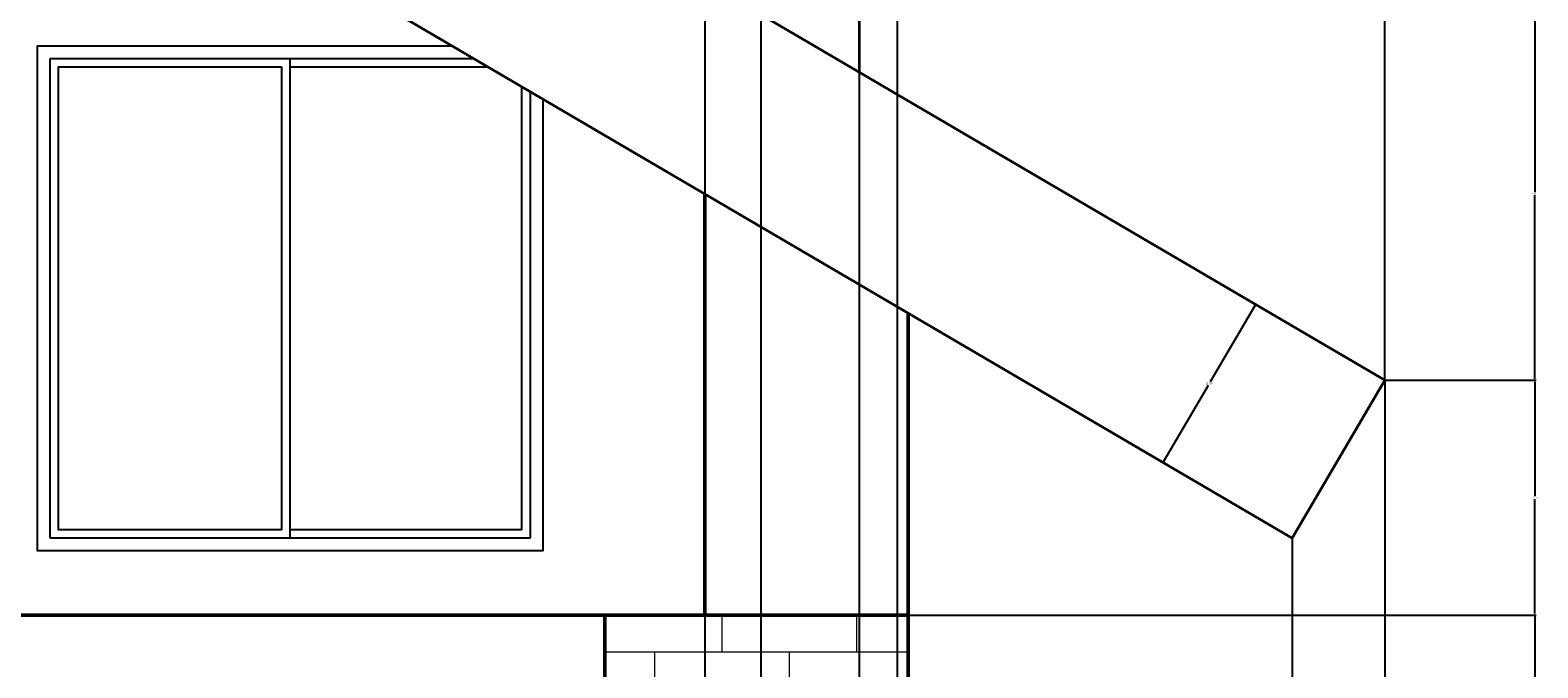
# Model space of a CAD drawing. Units: inches. Extents: x 27 to 409, y -26 to 294.
# Tile 6 of 7: x 230 to 409, y 102 to 178. Entities that reach past the tile are written whole.
import ezdxf

# ---------------------------------------------------------------- set-up
doc = ezdxf.new("R2010")
doc.units = ezdxf.units.IN
doc.header["$MEASUREMENT"] = 0
for name, color, linetype, lineweight in [('A-ANNO-DIMS', 2, 'Continuous', 18), ('A-GLAZ', 4, 'Continuous', 25), ('A-ROOF', 1, 'Continuous', 35), ('A-WALL', 7, 'Continuous', 50), ('A-WALL-PATT', 8, 'Continuous', 13)]:
    doc.layers.add(name, color=color, linetype=linetype, lineweight=lineweight)
doc.styles.get("Standard").update_dxf_attribs({"font": 'arial.ttf'})
doc.dimstyles.get("Standard").update_dxf_attribs({"dimtxt": 0.18, "dimasz": 0.18, "dimexe": 0.18, "dimexo": 0.0625, "dimgap": 0.09, "dimtad": 0, "dimtih": 1, "dimtoh": 1, "dimdec": 4, "dimzin": 0, "dimdsep": 46, "dimtxsty": 'Standard', "dimcen": 0.09, "dimadec": 0, "dimazin": 0, "dimtfac": 1, "dimtdec": 4, "dimtofl": 0, "dimtmove": 0, "dimatfit": 3, "dimfxl": 1, "dimtolj": 1, "dimtzin": 0, "dimarcsym": 0})

# ---------------------------------------------------------------- blocks, each defined once
blk = doc.blocks.new('*D7')
at = {"layer": 'A-ANNO-DIMS', "color": 0, "lineweight": -2, "transparency": 16777216}
for p, q in [((45.58, 108.44), (45.58, 293.63)), ((45.76, 293.45), (217.77, 293.45)), ((390.53, 293.45), (218.52, 293.45)), ((390.71, 136.32), (390.71, 293.63))]:
    blk.add_line(p, q, dxfattribs=at)
at = {"layer": 'A-ANNO-DIMS', "color": 0, "transparency": 16777216}
for points in [[(45.76, 293.48), (45.76, 293.42), (45.58, 293.45)], [(390.53, 293.48), (390.53, 293.42), (390.71, 293.45)]]:
    blk.add_solid(points, dxfattribs=at)
at = {"layer": 'Defpoints', "color": 0, "transparency": 16777216}
for p in [(390.71, 293.45), (390.71, 136.26), (45.58, 108.38)]:
    blk.add_point(p, dxfattribs=at)
at = {"layer": 'A-ANNO-DIMS', "color": 0, "transparency": 16777216, "insert": (218.14, 293.45), "char_height": 0.18, "attachment_point": 5}
blk.add_mtext('\\A1;345.1', dxfattribs=at)
blk = doc.blocks.new('*D20')
at = {"layer": 'A-ANNO-DIMS', "color": 0, "lineweight": -2, "transparency": 16777216}
for p, q in [((210.09, 143.71), (210.09, -26.5)), ((230.52, -8.58), (230.52, -26.5)), ((210.27, -26.32), (219.84, -26.32)), ((230.34, -26.32), (220.77, -26.32))]:
    blk.add_line(p, q, dxfattribs=at)
at = {"layer": 'A-ANNO-DIMS', "color": 0, "transparency": 16777216}
for points in [[(210.27, -26.29), (210.27, -26.35), (210.09, -26.32)], [(230.34, -26.29), (230.34, -26.35), (230.52, -26.32)]]:
    blk.add_solid(points, dxfattribs=at)
at = {"layer": 'Defpoints', "color": 0, "transparency": 16777216}
for p in [(210.09, 143.77), (230.52, -8.52), (230.52, -26.32)]:
    blk.add_point(p, dxfattribs=at)
at = {"layer": 'A-ANNO-DIMS', "color": 0, "transparency": 16777216, "insert": (220.31, -26.32), "char_height": 0.18, "attachment_point": 5}
blk.add_mtext('\\A1;20.435', dxfattribs=at)
blk = doc.blocks.new('*D21')
at = {"layer": 'A-ANNO-DIMS', "color": 0, "lineweight": -2, "transparency": 16777216}
for p, q in [((298.08, 108.32), (298.08, -26.5)), ((230.52, -8.58), (230.52, -26.5)), ((230.7, -26.32), (263.9, -26.32)), ((297.9, -26.32), (264.69, -26.32))]:
    blk.add_line(p, q, dxfattribs=at)
at = {"layer": 'A-ANNO-DIMS', "color": 0, "transparency": 16777216}
for points in [[(230.7, -26.29), (230.7, -26.35), (230.52, -26.32)], [(297.9, -26.29), (297.9, -26.35), (298.08, -26.32)]]:
    blk.add_solid(points, dxfattribs=at)
at = {"layer": 'Defpoints', "color": 0, "transparency": 16777216}
for p in [(298.08, 108.38), (230.52, -8.52), (298.08, -26.32)]:
    blk.add_point(p, dxfattribs=at)
at = {"layer": 'A-ANNO-DIMS', "color": 0, "transparency": 16777216, "insert": (264.3, -26.32), "char_height": 0.18, "attachment_point": 5}
blk.add_mtext('\\A1;67.55', dxfattribs=at)
blk = doc.blocks.new('*D22')
at = {"layer": 'A-ANNO-DIMS', "color": 0, "lineweight": -2, "transparency": 16777216}
for p, q in [((309.93, 158.34), (309.93, -26.5)), ((298.08, 108.32), (298.08, -26.5)), ((298.26, -26.32), (303.61, -26.32)), ((309.75, -26.32), (304.39, -26.32))]:
    blk.add_line(p, q, dxfattribs=at)
at = {"layer": 'A-ANNO-DIMS', "color": 0, "transparency": 16777216}
for points in [[(298.26, -26.29), (298.26, -26.35), (298.08, -26.32)], [(309.75, -26.29), (309.75, -26.35), (309.93, -26.32)]]:
    blk.add_solid(points, dxfattribs=at)
at = {"layer": 'Defpoints', "color": 0, "transparency": 16777216}
for p in [(309.93, 158.4), (298.08, 108.38), (309.93, -26.32)]:
    blk.add_point(p, dxfattribs=at)
at = {"layer": 'A-ANNO-DIMS', "color": 0, "transparency": 16777216, "insert": (304, -26.32), "char_height": 0.18, "attachment_point": 5}
blk.add_mtext('\\A1;11.85', dxfattribs=at)
blk = doc.blocks.new('*D23')
at = {"layer": 'A-ANNO-DIMS', "color": 0, "lineweight": -2, "transparency": 16777216}
for p, q in [((309.93, 158.34), (309.93, -26.5)), ((334.08, 15.42), (334.08, -26.5)), ((310.11, -26.32), (321.6, -26.32)), ((333.9, -26.32), (322.4, -26.32))]:
    blk.add_line(p, q, dxfattribs=at)
at = {"layer": 'A-ANNO-DIMS', "color": 0, "transparency": 16777216}
for points in [[(310.11, -26.29), (310.11, -26.35), (309.93, -26.32)], [(333.9, -26.29), (333.9, -26.35), (334.08, -26.32)]]:
    blk.add_solid(points, dxfattribs=at)
at = {"layer": 'Defpoints', "color": 0, "transparency": 16777216}
for p in [(309.93, 158.4), (334.08, 15.48), (334.08, -26.32)]:
    blk.add_point(p, dxfattribs=at)
at = {"layer": 'A-ANNO-DIMS', "color": 0, "transparency": 16777216, "insert": (322, -26.32), "char_height": 0.18, "attachment_point": 5}
blk.add_mtext('\\A1;24.15', dxfattribs=at)
blk = doc.blocks.new('*D24')
at = {"layer": 'A-ANNO-DIMS', "color": 0, "lineweight": -2, "transparency": 16777216}
for p, q in [((379.72, 117.44), (379.72, -26.5)), ((334.08, 15.42), (334.08, -26.5)), ((334.26, -26.32), (356.5, -26.32)), ((379.54, -26.32), (357.29, -26.32))]:
    blk.add_line(p, q, dxfattribs=at)
at = {"layer": 'A-ANNO-DIMS', "color": 0, "transparency": 16777216}
for points in [[(334.26, -26.29), (334.26, -26.35), (334.08, -26.32)], [(379.54, -26.29), (379.54, -26.35), (379.72, -26.32)]]:
    blk.add_solid(points, dxfattribs=at)
at = {"layer": 'Defpoints', "color": 0, "transparency": 16777216}
for p in [(379.72, 117.5), (334.08, 15.48), (379.72, -26.32)]:
    blk.add_point(p, dxfattribs=at)
at = {"layer": 'A-ANNO-DIMS', "color": 0, "transparency": 16777216, "insert": (356.9, -26.32), "char_height": 0.18, "attachment_point": 5}
blk.add_mtext('\\A1;45.64', dxfattribs=at)
blk = doc.blocks.new('*D25')
at = {"layer": 'A-ANNO-DIMS', "color": 0, "lineweight": -2, "transparency": 16777216}
for p, q in [((390.71, 136.19), (390.71, -26.5)), ((379.72, 117.44), (379.72, -26.5)), ((379.9, -26.32), (384.83, -26.32)), ((390.53, -26.32), (385.6, -26.32))]:
    blk.add_line(p, q, dxfattribs=at)
at = {"layer": 'A-ANNO-DIMS', "color": 0, "transparency": 16777216}
for points in [[(379.9, -26.29), (379.9, -26.35), (379.72, -26.32)], [(390.53, -26.29), (390.53, -26.35), (390.71, -26.32)]]:
    blk.add_solid(points, dxfattribs=at)
at = {"layer": 'Defpoints', "color": 0, "transparency": 16777216}
for p in [(390.71, 136.26), (379.72, 117.5), (390.71, -26.32)]:
    blk.add_point(p, dxfattribs=at)
at = {"layer": 'A-ANNO-DIMS', "color": 0, "transparency": 16777216, "insert": (385.21, -26.32), "char_height": 0.18, "attachment_point": 5}
blk.add_mtext('\\A1;10.99', dxfattribs=at)
blk = doc.blocks.new('*D42')
at = {"layer": 'A-ANNO-DIMS', "color": 0, "lineweight": -2, "transparency": 16777216}
for p, q in [((334.14, 108.38), (408.69, 108.38)), ((408.51, 108.2), (408.51, 62.11)), ((408.51, 15.66), (408.51, 61.75)), ((334.14, 15.48), (408.69, 15.48))]:
    blk.add_line(p, q, dxfattribs=at)
at = {"layer": 'A-ANNO-DIMS', "color": 0, "transparency": 16777216}
for points in [[(408.48, 108.2), (408.54, 108.2), (408.51, 108.38)], [(408.48, 15.66), (408.54, 15.66), (408.51, 15.48)]]:
    blk.add_solid(points, dxfattribs=at)
at = {"layer": 'Defpoints', "color": 0, "transparency": 16777216}
for p in [(334.08, 108.38), (408.51, 108.38), (334.08, 15.48)]:
    blk.add_point(p, dxfattribs=at)
at = {"layer": 'A-ANNO-DIMS', "color": 0, "transparency": 16777216, "insert": (408.51, 61.93), "char_height": 0.18, "attachment_point": 5}
blk.add_mtext('\\A1;92.9', dxfattribs=at)
blk = doc.blocks.new('*D43')
at = {"layer": 'A-ANNO-DIMS', "color": 0, "lineweight": -2, "transparency": 16777216}
for p, q in [((390.77, 136.26), (408.69, 136.26)), ((408.51, 136.08), (408.51, 122.5)), ((408.51, 108.56), (408.51, 122.14)), ((334.14, 108.38), (408.69, 108.38))]:
    blk.add_line(p, q, dxfattribs=at)
at = {"layer": 'A-ANNO-DIMS', "color": 0, "transparency": 16777216}
for points in [[(408.48, 136.08), (408.54, 136.08), (408.51, 136.26)], [(408.48, 108.56), (408.54, 108.56), (408.51, 108.38)]]:
    blk.add_solid(points, dxfattribs=at)
at = {"layer": 'Defpoints', "color": 0, "transparency": 16777216}
for p in [(390.71, 136.26), (408.51, 136.26), (334.08, 108.38)]:
    blk.add_point(p, dxfattribs=at)
at = {"layer": 'A-ANNO-DIMS', "color": 0, "transparency": 16777216, "insert": (408.51, 122.32), "char_height": 0.18, "attachment_point": 5}
blk.add_mtext('\\A1;27.877', dxfattribs=at)
blk = doc.blocks.new('*D44')
at = {"layer": 'A-ANNO-DIMS', "color": 0, "lineweight": -2, "transparency": 16777216}
for p, q in [((166.14, 180.59), (408.69, 180.59)), ((408.51, 180.41), (408.51, 158.6)), ((408.51, 136.44), (408.51, 158.24)), ((390.77, 136.26), (408.69, 136.26))]:
    blk.add_line(p, q, dxfattribs=at)
at = {"layer": 'A-ANNO-DIMS', "color": 0, "transparency": 16777216}
for points in [[(408.48, 180.41), (408.54, 180.41), (408.51, 180.59)], [(408.48, 136.44), (408.54, 136.44), (408.51, 136.26)]]:
    blk.add_solid(points, dxfattribs=at)
at = {"layer": 'Defpoints', "color": 0, "transparency": 16777216}
for p in [(166.08, 180.59), (408.51, 180.59), (390.71, 136.26)]:
    blk.add_point(p, dxfattribs=at)
at = {"layer": 'A-ANNO-DIMS', "color": 0, "transparency": 16777216, "insert": (408.51, 158.42), "char_height": 0.18, "attachment_point": 5}
blk.add_mtext('\\A1;44.33', dxfattribs=at)
blk = doc.blocks.new('*D52')
at = {"layer": 'A-ANNO-DIMS', "color": 0, "lineweight": -2, "transparency": 16777216}
for p, q in [((375.26, 145.1), (369.96, 136.06)), ((390.65, 136.29), (375.19, 145.35)), ((364.45, 126.66), (369.75, 135.7)), ((379.66, 117.54), (364.2, 126.59))]:
    blk.add_line(p, q, dxfattribs=at)
at = {"layer": 'A-ANNO-DIMS', "color": 0, "transparency": 16777216}
for points in [[(375.23, 145.12), (375.28, 145.09), (375.35, 145.26)], [(364.42, 126.67), (364.48, 126.64), (364.36, 126.5)]]:
    blk.add_solid(points, dxfattribs=at)
at = {"layer": 'Defpoints', "color": 0, "transparency": 16777216}
for p in [(375.35, 145.26), (390.71, 136.26), (379.72, 117.5)]:
    blk.add_point(p, dxfattribs=at)
at = {"layer": 'A-ANNO-DIMS', "color": 0, "transparency": 16777216, "insert": (369.85, 135.88), "char_height": 0.18, "attachment_point": 5}
blk.add_mtext('\\A1;21.736', dxfattribs=at)
blk = doc.blocks.new('*D82')
at = {"layer": 'A-ANNO-DIMS', "color": 0, "lineweight": -2, "transparency": 16777216}
for p, q in [((309.93, 228.32), (309.93, -26.5)), ((316.59, 228.32), (316.59, -26.5)), ((310.11, -26.32), (312.86, -26.32)), ((316.41, -26.32), (313.65, -26.32))]:
    blk.add_line(p, q, dxfattribs=at)
at = {"layer": 'A-ANNO-DIMS', "color": 0, "transparency": 16777216}
for points in [[(310.11, -26.29), (310.11, -26.35), (309.93, -26.32)], [(316.41, -26.29), (316.41, -26.35), (316.59, -26.32)]]:
    blk.add_solid(points, dxfattribs=at)
at = {"layer": 'Defpoints', "color": 0, "transparency": 16777216}
for p in [(309.93, 228.38), (316.59, 228.38), (316.59, -26.32)]:
    blk.add_point(p, dxfattribs=at)
at = {"layer": 'A-ANNO-DIMS', "color": 0, "transparency": 16777216, "insert": (313.26, -26.32), "char_height": 0.18, "attachment_point": 5}
blk.add_mtext('\\A1;6.665', dxfattribs=at)
blk = doc.blocks.new('*D83')
at = {"layer": 'A-ANNO-DIMS', "color": 0, "lineweight": -2, "transparency": 16777216}
for p, q in [((316.59, 228.32), (316.59, -26.5)), ((328.29, 228.32), (328.29, -26.5)), ((316.77, -26.32), (321.99, -26.32)), ((328.11, -26.32), (322.9, -26.32))]:
    blk.add_line(p, q, dxfattribs=at)
at = {"layer": 'A-ANNO-DIMS', "color": 0, "transparency": 16777216}
for points in [[(316.77, -26.29), (316.77, -26.35), (316.59, -26.32)], [(328.11, -26.29), (328.11, -26.35), (328.29, -26.32)]]:
    blk.add_solid(points, dxfattribs=at)
at = {"layer": 'Defpoints', "color": 0, "transparency": 16777216}
for p in [(316.59, 228.38), (328.29, 228.38), (328.29, -26.32)]:
    blk.add_point(p, dxfattribs=at)
at = {"layer": 'A-ANNO-DIMS', "color": 0, "transparency": 16777216, "insert": (322.44, -26.32), "char_height": 0.18, "attachment_point": 5}
blk.add_mtext('\\A1;11.699', dxfattribs=at)
blk = doc.blocks.new('*D84')
at = {"layer": 'A-ANNO-DIMS', "color": 0, "lineweight": -2, "transparency": 16777216}
for p, q in [((328.29, 228.32), (328.29, -26.5)), ((332.8, 228.32), (332.8, -26.5)), ((328.47, -26.32), (330.17, -26.32)), ((332.62, -26.32), (330.93, -26.32))]:
    blk.add_line(p, q, dxfattribs=at)
at = {"layer": 'A-ANNO-DIMS', "color": 0, "transparency": 16777216}
for points in [[(328.47, -26.29), (328.47, -26.35), (328.29, -26.32)], [(332.62, -26.29), (332.62, -26.35), (332.8, -26.32)]]:
    blk.add_solid(points, dxfattribs=at)
at = {"layer": 'Defpoints', "color": 0, "transparency": 16777216}
for p in [(328.29, 228.38), (332.8, 228.38), (332.8, -26.32)]:
    blk.add_point(p, dxfattribs=at)
at = {"layer": 'A-ANNO-DIMS', "color": 0, "transparency": 16777216, "insert": (330.55, -26.32), "char_height": 0.18, "attachment_point": 5}
blk.add_mtext('\\A1;4.511', dxfattribs=at)

msp = doc.modelspace()

# ---------------------------------------------------------------- hatches: boundary and pattern name
at = {"layer": 'A-WALL-PATT'}
h = msp.add_hatch(dxfattribs=at)
h.set_pattern_fill('AR-B816', color=256)
h.paths.add_polyline_path([(334.0751, 108.3803), (298.0751, 108.3803), (298.0751, 15.4825), (334.0751, 15.4825)])

# ---------------------------------------------------------------- linework, layer by layer
at = {"layer": 'A-GLAZ'}
for p, q in [((232.1845, 117.4951), (232.1845, 174.4951)), ((232.1845, 174.4951), (260.6845, 174.4951)), ((260.6845, 117.4951), (260.6845, 174.4951)), ((260.6845, 174.4951), (282.4614, 174.4951)), ((289.1845, 170.5554), (289.1845, 117.4951)), ((260.6845, 117.4951), (232.1845, 117.4951)), ((289.1845, 117.4951), (260.6845, 117.4951))]:
    msp.add_line(p, q, dxfattribs=at)
for points in [[(290.6845, 169.6764), (290.6845, 115.9951), (230.6845, 115.9951), (230.6845, 175.9951), (279.9017, 175.9951)], [(259.6845, 173.4952), (259.6845, 118.4951), (233.1845, 118.4951), (233.1845, 173.4951), (259.6845, 173.4951)], [(260.6845, 173.4951), (284.1679, 173.4951)], [(288.1845, 171.1414), (288.1845, 118.4951), (260.6845, 118.4951)]]:
    msp.add_lwpolyline(points, dxfattribs=at)
at = {"layer": 'A-ROOF'}
for points in [[(166.0751, 242.6981), (379.7157, 117.5036), (390.7054, 136.2572), (152.833, 275.6517)], [(309.9262, 228.3803), (328.2901, 228.3803), (328.2901, 172.8329)]]:
    msp.add_lwpolyline(points, dxfattribs=at)
at = {"layer": 'A-WALL'}
for p, q in [((309.9262, 108.3803), (309.9262, 158.4006)), ((334.0751, -8.5175), (334.0751, 135.4825)), ((229.1036, 108.3803), (334.0751, 108.3803)), ((298.0751, 15.4825), (298.0751, 108.3803))]:
    msp.add_line(p, q, dxfattribs=at)
msp.add_lwpolyline([(334.0751, 144.2493), (334.0751, 108.3803), (94.0751, 108.3803)], dxfattribs=at)

# ---------------------------------------------------------------- dimensions: what is measured, and where the dimension line sits
at = {"layer": 'A-ANNO-DIMS'}
for base, p1, p2, override, picture, middle in [((390.7054, 293.4517), (45.5772, 108.3803), (390.7054, 136.2572), {"dimdec": 1, "dimlfac": 1, "dimrnd": 0, "dimzin": 0, "dimdsep": 46, "dimlunit": 2}, '*D7', (218.1413, 293.4517)), ((316.5916, -26.3175), (309.9262, 228.3803), (316.5916, 228.3803), {"dimdec": 3, "dimlfac": 1, "dimrnd": 0, "dimzin": 0, "dimdsep": 46, "dimlunit": 2}, '*D82', (313.2589, -26.3175)), ((328.29013, -26.31755), (316.59157, 228.38031), (328.29013, 228.38031), {"dimdec": 3, "dimlfac": 1, "dimrnd": 0, "dimzin": 0, "dimdsep": 46, "dimlunit": 2}, '*D83', (322.44085, -26.31755)), ((332.8007, -26.3175), (328.2901, 228.3803), (332.8007, 228.3803), {"dimdec": 3, "dimlfac": 1, "dimrnd": 0, "dimzin": 0, "dimdsep": 46, "dimlunit": 2}, '*D84', (330.5454, -26.3175)), ((309.9262, -26.3175), (298.0751, 108.3803), (309.9262, 158.4006), {"dimdec": 2, "dimlfac": 1, "dimrnd": 0, "dimzin": 0, "dimdsep": 46, "dimlunit": 2}, '*D22', (304.0006, -26.3175)), ((334.0751, -26.3175), (309.9262, 158.4006), (334.0751, 15.4825), {"dimdec": 2, "dimlfac": 1, "dimrnd": 0, "dimzin": 0, "dimdsep": 46, "dimlunit": 2}, '*D23', (322.0006, -26.3175)), ((230.5245, -26.3175), (210.0897, 143.7732), (230.5245, -8.5175), {"dimdec": 3, "dimlfac": 1, "dimrnd": 0, "dimzin": 0, "dimdsep": 46, "dimlunit": 2}, '*D20', (220.3071, -26.3175)), ((390.7054, -26.3175), (379.7157, 117.5036), (390.7054, 136.2572), {"dimdec": 2, "dimlfac": 1, "dimrnd": 0, "dimzin": 0, "dimdsep": 46, "dimlunit": 2}, '*D25', (385.2106, -26.3175)), ((379.7157, -26.3175), (334.0751, 15.4825), (379.7157, 117.5036), {"dimdec": 2, "dimlfac": 1, "dimrnd": 0, "dimzin": 0, "dimdsep": 46, "dimlunit": 2}, '*D24', (356.8954, -26.3175)), ((298.0751, -26.3175), (230.5245, -8.5175), (298.0751, 108.3803), {"dimdec": 2, "dimlfac": 1, "dimrnd": 0, "dimzin": 0, "dimdsep": 46, "dimlunit": 2}, '*D21', (264.2998, -26.3175))]:
    dim = msp.add_linear_dim(base=base, p1=p1, p2=p2, dimstyle='Standard', override=override, dxfattribs=at)
    dim.commit()
    dim.dimension.update_dxf_attribs({"geometry": picture, "text_midpoint": middle})
for base, p1, p2, angle, override, picture, middle in [((408.5054, 180.5852), (390.7054, 136.2572), (166.0751, 180.5852), 90, {"dimdec": 2, "dimlfac": 1, "dimrnd": 0, "dimzin": 0, "dimdsep": 46, "dimlunit": 2}, '*D44', (408.5054, 158.4212)), ((375.3481, 145.2567), (379.7157, 117.5036), (390.7054, 136.2572), 59.629482, {"dimdec": 3, "dimlfac": 1, "dimrnd": 0, "dimzin": 0, "dimdsep": 46, "dimlunit": 2}, '*D52', (369.8532, 135.8799)), ((408.5054, 136.2572), (334.0751, 108.3803), (390.7054, 136.2572), 90, {"dimdec": 3, "dimlfac": 1, "dimrnd": 0, "dimzin": 0, "dimdsep": 46, "dimlunit": 2}, '*D43', (408.5054, 122.3188)), ((408.5054, 108.3803), (334.0751, 15.4825), (334.0751, 108.3803), 90, {"dimdec": 1, "dimlfac": 1, "dimrnd": 0, "dimzin": 0, "dimdsep": 46, "dimlunit": 2}, '*D42', (408.5054, 61.9314))]:
    dim = msp.add_linear_dim(base=base, p1=p1, p2=p2, angle=angle, dimstyle='Standard', override=override, dxfattribs=at)
    dim.commit()
    dim.dimension.update_dxf_attribs({"geometry": picture, "text_midpoint": middle})

doc.saveas('drawing.dxf')
